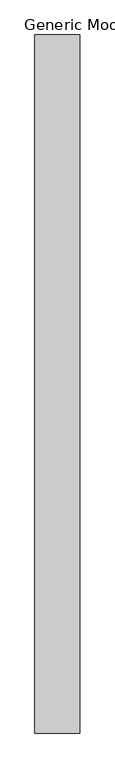
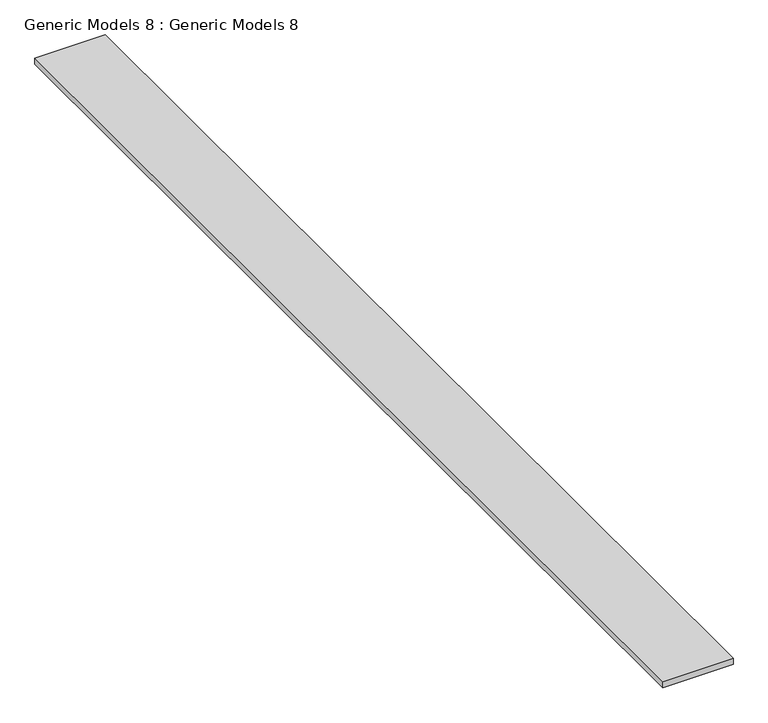
"""IFC4 building model written with IfcOpenShell, lengths in millimetres: proxy geometry, Generic Models 8 : Generic Models 8."""

from ifc_helpers import new_model, si_unit, frame, origin, place, context, project, spatial, polyline, outline, extrude, source, transform, mapped, element, save


def generic_models_8_generic_models_8_d6955511(model_context):
    return source(origin(), model_context, "Body", "SweptSolid", [
        extrude(outline(polyline([(9452.9373895, -10195.4484681), (9452.9373895, 15703.0562567), (11124.0222236, 15703.0562567), (11124.0222236, -10195.4484681), (9452.9373895, -10195.4484681)])), frame((0.0, 0.0, -152.4), z_axis=(0.0, 0.0, 1.0), x_axis=(1.0, 0.0, 0.0)), (0.0, 0.0, 1.0), 152.4),
    ])


if __name__ == "__main__":
    model = new_model("IFC4")
    model_context = context("Model", 3, world=origin())
    ifc_project = project(units=[si_unit("LENGTHUNIT", "METRE", prefix="MILLI")], contexts=[model_context])
    site = spatial("IfcSite", under=ifc_project)
    building = spatial("IfcBuilding", under=site)
    placement = place(None, origin())
    generic_models_8_generic_models_8_shape = generic_models_8_generic_models_8_d6955511(model_context)
    element("IfcBuildingElementProxy", 1, Name="Generic Models 8 : Generic Models 8", ObjectType="Generic Models 8 : Generic Models 8", at=placement, inside=building, context=model_context, shape_type="MappedRepresentation", body=[
        mapped(generic_models_8_generic_models_8_shape, transform((0.0, 0.0, 0.0), x_axis=(1.0, 0.0, 0.0), y_axis=(0.0, 1.0, 0.0), z_axis=(0.0, 0.0, 1.0))),
    ])
    save(model, "model.ifc")
